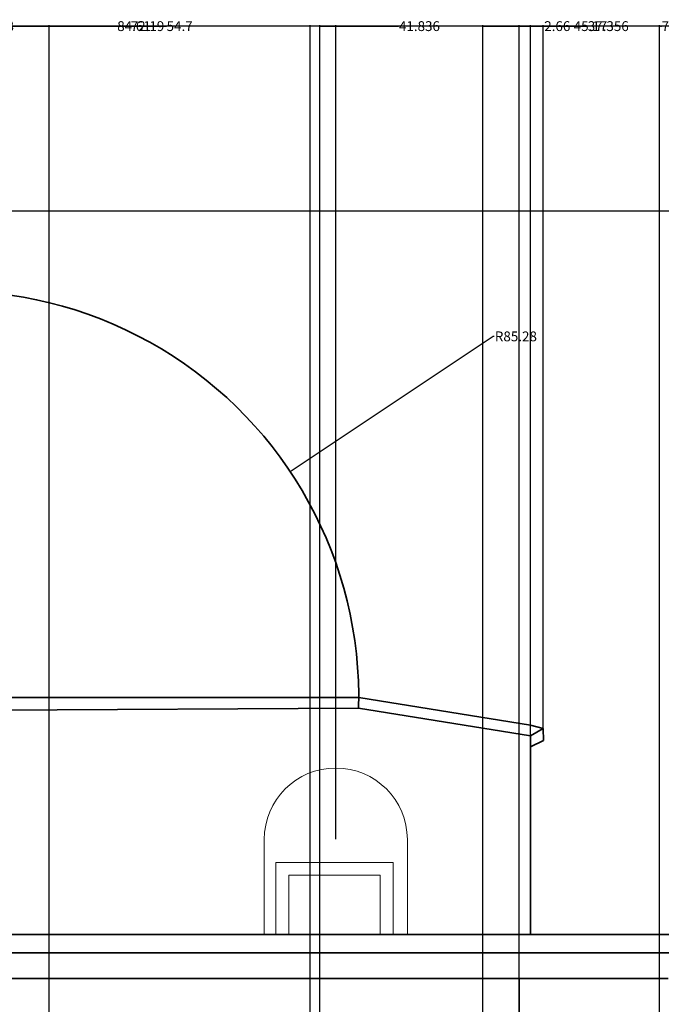
# Model space of a CAD drawing. Units: inches. Extents: x 14 to 859, y 52 to 711.
# Tile 9 of 11: x 442 to 577, y 504 to 711. Entities that reach past the tile are written whole.
import ezdxf

# ---------------------------------------------------------------- set-up
doc = ezdxf.new("R2010")
doc.units = ezdxf.units.IN
doc.header["$MEASUREMENT"] = 0
for name, color, linetype, lineweight in [('A-ANNO-DIMS', 2, 'Continuous', 18), ('A-ELEV', 7, 'Continuous', 35), ('A-GLAZ', 4, 'Continuous', 18), ('A-ROOF', 7, 'Continuous', 35)]:
    doc.layers.add(name, color=color, linetype=linetype, lineweight=lineweight)
doc.styles.get("Standard").update_dxf_attribs({"font": 'arial.ttf'})
doc.dimstyles.get("Standard").update_dxf_attribs({"dimtxt": 2.0625, "dimasz": 0.18, "dimexe": 0.18, "dimexo": 0.0625, "dimgap": 0.09, "dimtad": 0, "dimtih": 1, "dimtoh": 1, "dimdec": 4, "dimzin": 0, "dimdsep": 46, "dimlunit": 4, "dimtxsty": 'Standard', "dimcen": 0.09, "dimadec": 0, "dimazin": 0, "dimtfac": 1, "dimtdec": 4, "dimtofl": 0, "dimtmove": 0, "dimatfit": 3, "dimfxl": 1, "dimtolj": 1, "dimtzin": 0, "dimarcsym": 0})

# ---------------------------------------------------------------- blocks, each defined once
blk = doc.blocks.new('WIN-DRUM-ARCHED')
for p, q in [((329.67, 519.05), (329.67, 538.94)), ((359.68, 519.05), (359.68, 538.94))]:
    blk.add_line(p, q)
for points in [[(332.09, 519.05), (332.09, 534.15), (356.71, 534.15), (356.71, 519.05)], [(334.8, 519.05), (334.8, 531.45), (354.01, 531.45), (354.01, 519.05)]]:
    blk.add_lwpolyline(points)
blk.add_arc((344.68, 538.94), 15, 0, 180)
blk = doc.blocks.new('*D13')
at = {"layer": 'A-ANNO-DIMS', "color": 0, "lineweight": -2, "transparency": 16777216}
for p, q in [((60.78, 339.73), (60.78, 709.71)), ((60.96, 709.53), (432.6, 709.53)), ((811.37, 709.53), (439.73, 709.53)), ((811.55, 339.73), (811.55, 709.71))]:
    blk.add_line(p, q, dxfattribs=at)
at = {"layer": 'A-ANNO-DIMS', "color": 0, "transparency": 16777216}
for points in [[(60.96, 709.56), (60.96, 709.5), (60.78, 709.53)], [(811.37, 709.56), (811.37, 709.5), (811.55, 709.53)]]:
    blk.add_solid(points, dxfattribs=at)
at = {"layer": 'Defpoints', "color": 0, "transparency": 16777216}
for p in [(811.55, 709.53), (60.78, 339.66), (811.55, 339.66)]:
    blk.add_point(p, dxfattribs=at)
at = {"layer": 'A-ANNO-DIMS', "color": 0, "transparency": 16777216, "insert": (436.17, 709.53), "char_height": 2.062, "attachment_point": 5}
blk.add_mtext('\\A1;750.8', dxfattribs=at)
blk = doc.blocks.new('*D19')
at = {"layer": 'A-ANNO-DIMS', "color": 0, "lineweight": -2, "transparency": 16777216}
for p, q in [((430.09, 670.76), (854.64, 670.76)), ((854.46, 670.58), (854.46, 538.71)), ((854.46, 404.55), (854.46, 536.42)), ((609.81, 404.37), (854.64, 404.37))]:
    blk.add_line(p, q, dxfattribs=at)
at = {"layer": 'A-ANNO-DIMS', "color": 0, "transparency": 16777216}
for points in [[(854.43, 670.58), (854.49, 670.58), (854.46, 670.76)], [(854.43, 404.55), (854.49, 404.55), (854.46, 404.37)]]:
    blk.add_solid(points, dxfattribs=at)
at = {"layer": 'Defpoints', "color": 0, "transparency": 16777216}
for p in [(430.02, 670.76), (854.46, 670.76), (609.75, 404.37)]:
    blk.add_point(p, dxfattribs=at)
at = {"layer": 'A-ANNO-DIMS', "color": 0, "transparency": 16777216, "insert": (854.46, 537.57), "char_height": 2.062, "attachment_point": 5}
blk.add_mtext('\\A1;266.4', dxfattribs=at)
blk = doc.blocks.new('*D22')
at = {"layer": 'A-ANNO-DIMS', "color": 0, "lineweight": -2, "transparency": 16777216}
for p, q in [((298.73, 341.73), (298.73, 709.71)), ((298.91, 709.53), (434.03, 709.53)), ((576.33, 709.53), (441.21, 709.53)), ((576.51, 341.73), (576.51, 709.71))]:
    blk.add_line(p, q, dxfattribs=at)
at = {"layer": 'A-ANNO-DIMS', "color": 0, "transparency": 16777216}
for points in [[(298.91, 709.56), (298.91, 709.5), (298.73, 709.53)], [(576.33, 709.56), (576.33, 709.5), (576.51, 709.53)]]:
    blk.add_solid(points, dxfattribs=at)
at = {"layer": 'Defpoints', "color": 0, "transparency": 16777216}
for p in [(576.51, 709.53), (298.73, 341.67), (576.51, 341.67)]:
    blk.add_point(p, dxfattribs=at)
at = {"layer": 'A-ANNO-DIMS', "color": 0, "transparency": 16777216, "insert": (437.62, 709.53), "char_height": 2.062, "attachment_point": 5}
blk.add_mtext('\\A1;277.8', dxfattribs=at)
blk = doc.blocks.new('*D23')
at = {"layer": 'A-ANNO-DIMS', "color": 0, "lineweight": -2, "transparency": 16777216}
for p, q in [((576.51, 341.73), (576.51, 709.71)), ((576.69, 709.53), (576.9, 709.53)), ((584.26, 709.53), (584.04, 709.53)), ((584.44, 352.49), (584.44, 709.71))]:
    blk.add_line(p, q, dxfattribs=at)
at = {"layer": 'A-ANNO-DIMS', "color": 0, "transparency": 16777216}
for points in [[(576.69, 709.56), (576.69, 709.5), (576.51, 709.53)], [(584.26, 709.56), (584.26, 709.5), (584.44, 709.53)]]:
    blk.add_solid(points, dxfattribs=at)
at = {"layer": 'Defpoints', "color": 0, "transparency": 16777216}
for p in [(584.44, 709.53), (584.44, 352.43), (576.51, 341.67)]:
    blk.add_point(p, dxfattribs=at)
at = {"layer": 'A-ANNO-DIMS', "color": 0, "transparency": 16777216, "insert": (580.47, 709.53), "char_height": 2.062, "attachment_point": 5}
blk.add_mtext('\\A1;7.935', dxfattribs=at)
blk = doc.blocks.new('*D98')
at = {"layer": 'A-ANNO-DIMS', "color": 0, "lineweight": -2, "transparency": 16777216}
for p, q in [((433.06, 447.01), (433.06, 709.71)), ((433.24, 709.53), (465.59, 709.53)), ((505.07, 709.53), (472.72, 709.53)), ((505.25, 447.01), (505.25, 709.71))]:
    blk.add_line(p, q, dxfattribs=at)
at = {"layer": 'A-ANNO-DIMS', "color": 0, "transparency": 16777216}
for points in [[(433.24, 709.56), (433.24, 709.5), (433.06, 709.53)], [(505.07, 709.56), (505.07, 709.5), (505.25, 709.53)]]:
    blk.add_solid(points, dxfattribs=at)
at = {"layer": 'Defpoints', "color": 0, "transparency": 16777216}
for p in [(505.25, 709.53), (433.06, 446.95), (505.25, 446.95)]:
    blk.add_point(p, dxfattribs=at)
at = {"layer": 'A-ANNO-DIMS', "color": 0, "transparency": 16777216, "insert": (469.15, 709.53), "char_height": 2.062, "attachment_point": 5}
blk.add_mtext('\\A1;72.19', dxfattribs=at)
blk = doc.blocks.new('*D99')
at = {"layer": 'A-ANNO-DIMS', "color": 0, "lineweight": -2, "transparency": 16777216}
for p, q in [((505.25, 447.01), (505.25, 709.71)), ((505.43, 709.53), (521.76, 709.53)), ((546.91, 709.53), (530.58, 709.53)), ((547.09, 509.85), (547.09, 709.71))]:
    blk.add_line(p, q, dxfattribs=at)
at = {"layer": 'A-ANNO-DIMS', "color": 0, "transparency": 16777216}
for points in [[(505.43, 709.56), (505.43, 709.5), (505.25, 709.53)], [(546.91, 709.56), (546.91, 709.5), (547.09, 709.53)]]:
    blk.add_solid(points, dxfattribs=at)
at = {"layer": 'Defpoints', "color": 0, "transparency": 16777216}
for p in [(547.09, 709.53), (547.09, 509.79), (505.25, 446.95)]:
    blk.add_point(p, dxfattribs=at)
at = {"layer": 'A-ANNO-DIMS', "color": 0, "transparency": 16777216, "insert": (526.17, 709.53), "char_height": 2.062, "attachment_point": 5}
blk.add_mtext('\\A1;41.836', dxfattribs=at)
blk = doc.blocks.new('*D100')
at = {"layer": 'A-ANNO-DIMS', "color": 0, "lineweight": -2, "transparency": 16777216}
for p, q in [((547.09, 509.85), (547.09, 709.71)), ((547.27, 709.53), (561.39, 709.53)), ((584.26, 709.53), (570.13, 709.53)), ((584.44, 504.44), (584.44, 709.71))]:
    blk.add_line(p, q, dxfattribs=at)
at = {"layer": 'A-ANNO-DIMS', "color": 0, "transparency": 16777216}
for points in [[(547.27, 709.56), (547.27, 709.5), (547.09, 709.53)], [(584.26, 709.56), (584.26, 709.5), (584.44, 709.53)]]:
    blk.add_solid(points, dxfattribs=at)
at = {"layer": 'Defpoints', "color": 0, "transparency": 16777216}
for p in [(584.44, 709.53), (547.09, 509.79), (584.44, 504.38)]:
    blk.add_point(p, dxfattribs=at)
at = {"layer": 'A-ANNO-DIMS', "color": 0, "transparency": 16777216, "insert": (565.76, 709.53), "char_height": 2.062, "attachment_point": 5}
blk.add_mtext('\\A1;37.356', dxfattribs=at)
blk = doc.blocks.new('*D105')
at = {"layer": 'A-ANNO-DIMS', "color": 0, "lineweight": -2, "transparency": 16777216}
for p, q in [((306.86, 560.74), (306.86, 709.71)), ((307.04, 709.53), (424.56, 709.53)), ((549.26, 709.53), (431.74, 709.53)), ((549.44, 560.74), (549.44, 709.71))]:
    blk.add_line(p, q, dxfattribs=at)
at = {"layer": 'A-ANNO-DIMS', "color": 0, "transparency": 16777216}
for points in [[(307.04, 709.56), (307.04, 709.5), (306.86, 709.53)], [(549.26, 709.56), (549.26, 709.5), (549.44, 709.53)]]:
    blk.add_solid(points, dxfattribs=at)
at = {"layer": 'Defpoints', "color": 0, "transparency": 16777216}
for p in [(549.44, 709.53), (306.86, 560.68), (549.44, 560.68)]:
    blk.add_point(p, dxfattribs=at)
at = {"layer": 'A-ANNO-DIMS', "color": 0, "transparency": 16777216, "insert": (428.15, 709.53), "char_height": 2.062, "attachment_point": 5}
blk.add_mtext('\\A1;242.6', dxfattribs=at)
blk = doc.blocks.new('*D107')
at = {"layer": 'A-ANNO-DIMS', "color": 0, "lineweight": -2, "transparency": 16777216}
for p, q in [((549.44, 560.74), (549.44, 709.71)), ((549.62, 709.53), (551.92, 709.53)), ((552.1, 562.26), (552.1, 709.71)), ((552.1, 709.53), (552.28, 709.53))]:
    blk.add_line(p, q, dxfattribs=at)
at = {"layer": 'A-ANNO-DIMS', "color": 0, "transparency": 16777216}
for points in [[(549.62, 709.56), (549.62, 709.5), (549.44, 709.53)], [(551.92, 709.56), (551.92, 709.5), (552.1, 709.53)]]:
    blk.add_solid(points, dxfattribs=at)
at = {"layer": 'Defpoints', "color": 0, "transparency": 16777216}
for p in [(552.1, 709.53), (552.1, 562.2), (549.44, 560.68)]:
    blk.add_point(p, dxfattribs=at)
at = {"layer": 'A-ANNO-DIMS', "color": 0, "transparency": 16777216, "insert": (555.07, 709.53), "char_height": 2.062, "attachment_point": 5}
blk.add_mtext('\\A1;2.66', dxfattribs=at)
blk = doc.blocks.new('*D112')
at = {"layer": 'A-ANNO-DIMS', "color": 0, "lineweight": -2, "transparency": 16777216}
for p, q in [((424.02, 539), (424.02, 709.71)), ((424.2, 709.53), (462.95, 709.53)), ((508.45, 709.53), (469.7, 709.53)), ((508.63, 539), (508.63, 709.71))]:
    blk.add_line(p, q, dxfattribs=at)
at = {"layer": 'A-ANNO-DIMS', "color": 0, "transparency": 16777216}
for points in [[(424.2, 709.56), (424.2, 709.5), (424.02, 709.53)], [(508.45, 709.56), (508.45, 709.5), (508.63, 709.53)]]:
    blk.add_solid(points, dxfattribs=at)
at = {"layer": 'Defpoints', "color": 0, "transparency": 16777216}
for p in [(508.63, 709.53), (424.02, 538.94), (508.63, 538.94)]:
    blk.add_point(p, dxfattribs=at)
at = {"layer": 'A-ANNO-DIMS', "color": 0, "transparency": 16777216, "insert": (466.32, 709.53), "char_height": 2.062, "attachment_point": 5}
blk.add_mtext('\\A1;84.61', dxfattribs=at)
blk = doc.blocks.new('*D121')
at = {"layer": 'A-ANNO-DIMS', "color": 0, "lineweight": -2, "transparency": 16777216}
for p, q in [((390.73, 404.43), (390.73, 709.71)), ((390.91, 709.53), (416.86, 709.53)), ((448.36, 709.53), (422.4, 709.53)), ((448.54, 404.43), (448.54, 709.71))]:
    blk.add_line(p, q, dxfattribs=at)
at = {"layer": 'A-ANNO-DIMS', "color": 0, "transparency": 16777216}
for points in [[(390.91, 709.56), (390.91, 709.5), (390.73, 709.53)], [(448.36, 709.56), (448.36, 709.5), (448.54, 709.53)]]:
    blk.add_solid(points, dxfattribs=at)
at = {"layer": 'Defpoints', "color": 0, "transparency": 16777216}
for p in [(448.54, 709.53), (390.73, 404.37), (448.54, 404.37)]:
    blk.add_point(p, dxfattribs=at)
at = {"layer": 'A-ANNO-DIMS', "color": 0, "transparency": 16777216, "insert": (419.63, 709.53), "char_height": 2.062, "attachment_point": 5}
blk.add_mtext('\\A1;57.8', dxfattribs=at)
blk = doc.blocks.new('*D122')
at = {"layer": 'A-ANNO-DIMS', "color": 0, "lineweight": -2, "transparency": 16777216}
for p, q in [((448.54, 404.43), (448.54, 709.71)), ((448.72, 709.53), (473.12, 709.53)), ((503.05, 709.53), (478.65, 709.53)), ((503.23, 404.43), (503.23, 709.71))]:
    blk.add_line(p, q, dxfattribs=at)
at = {"layer": 'A-ANNO-DIMS', "color": 0, "transparency": 16777216}
for points in [[(448.72, 709.56), (448.72, 709.5), (448.54, 709.53)], [(503.05, 709.56), (503.05, 709.5), (503.23, 709.53)]]:
    blk.add_solid(points, dxfattribs=at)
at = {"layer": 'Defpoints', "color": 0, "transparency": 16777216}
for p in [(503.23, 709.53), (448.54, 404.37), (503.23, 404.37)]:
    blk.add_point(p, dxfattribs=at)
at = {"layer": 'A-ANNO-DIMS', "color": 0, "transparency": 16777216, "insert": (475.89, 709.53), "char_height": 2.062, "attachment_point": 5}
blk.add_mtext('\\A1;54.7', dxfattribs=at)
blk = doc.blocks.new('*D123')
at = {"layer": 'A-ANNO-DIMS', "color": 0, "lineweight": -2, "transparency": 16777216}
for p, q in [((539.45, 404.43), (539.45, 709.71)), ((539.63, 709.53), (558.42, 709.53)), ((584.44, 709.53), (565.64, 709.53)), ((584.62, 404.43), (584.62, 709.71))]:
    blk.add_line(p, q, dxfattribs=at)
at = {"layer": 'A-ANNO-DIMS', "color": 0, "transparency": 16777216}
for points in [[(539.63, 709.56), (539.63, 709.5), (539.45, 709.53)], [(584.44, 709.56), (584.44, 709.5), (584.62, 709.53)]]:
    blk.add_solid(points, dxfattribs=at)
at = {"layer": 'Defpoints', "color": 0, "transparency": 16777216}
for p in [(584.62, 709.53), (539.45, 404.37), (584.62, 404.37)]:
    blk.add_point(p, dxfattribs=at)
at = {"layer": 'A-ANNO-DIMS', "color": 0, "transparency": 16777216, "insert": (562.03, 709.53), "char_height": 2.062, "attachment_point": 5}
blk.add_mtext('\\A1;45.17', dxfattribs=at)
blk = doc.blocks.new('*D130')
at = {"layer": 'A-ANNO-DIMS', "color": 0, "lineweight": -2, "transparency": 16777216}
for p, q in [((541.65, 644.46), (499.24, 616.16)), ((541.83, 644.46), (541.65, 644.46)), ((428.06, 568.74), (428.24, 568.74)), ((428.15, 568.65), (428.15, 568.83))]:
    blk.add_line(p, q, dxfattribs=at)
at = {"layer": 'A-ANNO-DIMS', "color": 0, "transparency": 16777216}
blk.add_solid([(499.22, 616.19), (499.26, 616.14), (499.09, 616.06)], dxfattribs=at)
at = {"layer": 'Defpoints', "color": 0, "transparency": 16777216}
for p in [(499.09, 616.06), (428.15, 568.74)]:
    blk.add_point(p, dxfattribs=at)
at = {"layer": 'A-ANNO-DIMS', "color": 0, "transparency": 16777216, "insert": (546.39, 644.46), "char_height": 2.062, "attachment_point": 5}
blk.add_mtext('\\A1;R85.28', dxfattribs=at)

msp = doc.modelspace()

# ---------------------------------------------------------------- linework, layer by layer
at = {"layer": 'A-ELEV'}
for p, q in [((434.8803, 568.7358), (513.4296, 568.7358)), ((549.4731, 562.9495), (513.4296, 568.7358)), ((434.8803, 566.0314), (513.3994, 566.4671)), ((549.4429, 560.6808), (513.3994, 566.4671)), ((552.1026, 562.1978), (549.4429, 560.6808)), ((549.4731, 562.9495), (552.1026, 562.1978)), ((552.1026, 562.1978), (552.1565, 559.7188)), ((549.4429, 560.6808), (549.4429, 519.0512)), ((552.1565, 559.7188), (549.4429, 558.4055)), ((264.6274, 519.0512), (555.2103, 519.0512)), ((555.2103, 519.0512), (598.9032, 519.0512)), ((276.5038, 515.1991), (537.6873, 515.1991)), ((537.6873, 515.1991), (588.3297, 515.1991)), ((276.5038, 509.7903), (537.6873, 509.7903)), ((537.6873, 509.7903), (578.3064, 509.7903)), ((547.0851, 405.9412), (547.0851, 509.7903))]:
    msp.add_line(p, q, dxfattribs=at)
at = {"layer": 'A-ROOF'}
msp.add_arc((428.1517, 568.7358), 85.2778, 358.475544, 180, dxfattribs=at)

# ---------------------------------------------------------------- block references
at = {"layer": 'A-GLAZ'}
msp.add_blockref('WIN-DRUM-ARCHED', (163.9522, 0), dxfattribs=at)

# ---------------------------------------------------------------- dimensions: what is measured, and where the dimension line sits
at = {"layer": 'A-ANNO-DIMS'}
for base, p1, p2, override, picture, middle in [((811.5534, 709.5262), (60.7804, 339.6626), (811.5534, 339.6626), {"dimdec": 1, "dimlfac": 1, "dimrnd": 0, "dimzin": 0, "dimdsep": 46, "dimlunit": 2}, '*D13', (436.1669, 709.5262)), ((576.5058, 709.5262), (298.7295, 341.6716), (576.5058, 341.6716), {"dimdec": 1, "dimlfac": 1, "dimrnd": 0, "dimzin": 0, "dimdsep": 46, "dimlunit": 2}, '*D22', (437.6176, 709.5262)), ((549.4429, 709.5262), (306.8606, 560.6808), (549.4429, 560.6808), {"dimdec": 1, "dimlfac": 1, "dimrnd": 0, "dimzin": 0, "dimdsep": 46, "dimlunit": 2}, '*D105', (428.1517, 709.5262)), ((448.5359, 709.5262), (390.7307, 404.3712), (448.5359, 404.3712), {"dimdec": 1, "dimlfac": 1, "dimrnd": 0, "dimzin": 0, "dimdsep": 46, "dimlunit": 2}, '*D121', (419.6333, 709.5262)), ((508.63, 709.5262), (424.0193, 538.9419), (508.63, 538.9419), {"dimdec": 2, "dimlfac": 1, "dimrnd": 0, "dimzin": 0, "dimdsep": 46, "dimlunit": 2}, '*D112', (466.3247, 709.5262)), ((505.2493, 709.5262), (433.06, 446.9501), (505.2493, 446.9501), {"dimdec": 2, "dimlfac": 1, "dimrnd": 0, "dimzin": 0, "dimdsep": 46, "dimlunit": 2}, '*D98', (469.1547, 709.5262)), ((503.2347, 709.5262), (448.5359, 404.3712), (503.2347, 404.3712), {"dimdec": 1, "dimlfac": 1, "dimrnd": 0, "dimzin": 0, "dimdsep": 46, "dimlunit": 2}, '*D122', (475.8853, 709.5262)), ((547.0851, 709.5262), (505.2493, 446.9501), (547.0851, 509.7903), {"dimdec": 3, "dimlfac": 1, "dimrnd": 0, "dimzin": 0, "dimdsep": 46, "dimlunit": 2}, '*D99', (526.1672, 709.5262)), ((584.619, 709.5262), (539.446, 404.3712), (584.619, 404.3712), {"dimdec": 2, "dimlfac": 1, "dimrnd": 0, "dimzin": 0, "dimdsep": 46, "dimlunit": 2}, '*D123', (562.0325, 709.5262)), ((584.4409, 709.5262), (547.0851, 509.7903), (584.4409, 504.3815), {"dimdec": 3, "dimlfac": 1, "dimrnd": 0, "dimzin": 0, "dimdsep": 46, "dimlunit": 2}, '*D100', (565.763, 709.5262)), ((552.1026, 709.5262), (549.4429, 560.6808), (552.1026, 562.1978), {"dimdec": 2, "dimlfac": 1, "dimrnd": 0, "dimzin": 0, "dimdsep": 46, "dimlunit": 2}, '*D107', (555.0682, 709.5262)), ((584.4409, 709.5262), (576.5058, 341.6716), (584.4409, 352.4291), {"dimdec": 3, "dimlfac": 1, "dimrnd": 0, "dimzin": 0, "dimdsep": 46, "dimlunit": 2}, '*D23', (580.4733, 709.5262))]:
    dim = msp.add_linear_dim(base=base, p1=p1, p2=p2, dimstyle='Standard', override=override, dxfattribs=at)
    dim.commit()
    dim.dimension.update_dxf_attribs({"geometry": picture, "text_midpoint": middle})
dim = msp.add_linear_dim(base=(854.4554, 670.7637), p1=(609.7501, 404.3712), p2=(430.0228, 670.7637), angle=90, dimstyle='Standard', override={"dimdec": 1, "dimlfac": 1, "dimrnd": 0, "dimzin": 0, "dimdsep": 46, "dimlunit": 2}, dxfattribs=at)
dim.commit()
dim.dimension.update_dxf_attribs({"geometry": '*D19', "text_midpoint": (854.4554, 537.5675)})
dim = msp.add_radius_dim(center=(428.1517, 568.7358), mpoint=(499.0902, 616.0649), dimstyle='Standard', override={"dimdec": 2, "dimlfac": 1, "dimrnd": 0, "dimzin": 0, "dimdsep": 46, "dimlunit": 2}, dxfattribs=at)
dim.commit()
dim.dimension.update_dxf_attribs({"geometry": '*D130', "text_midpoint": (546.3923, 644.4623), "dimtype": 164})

doc.saveas('drawing.dxf')
